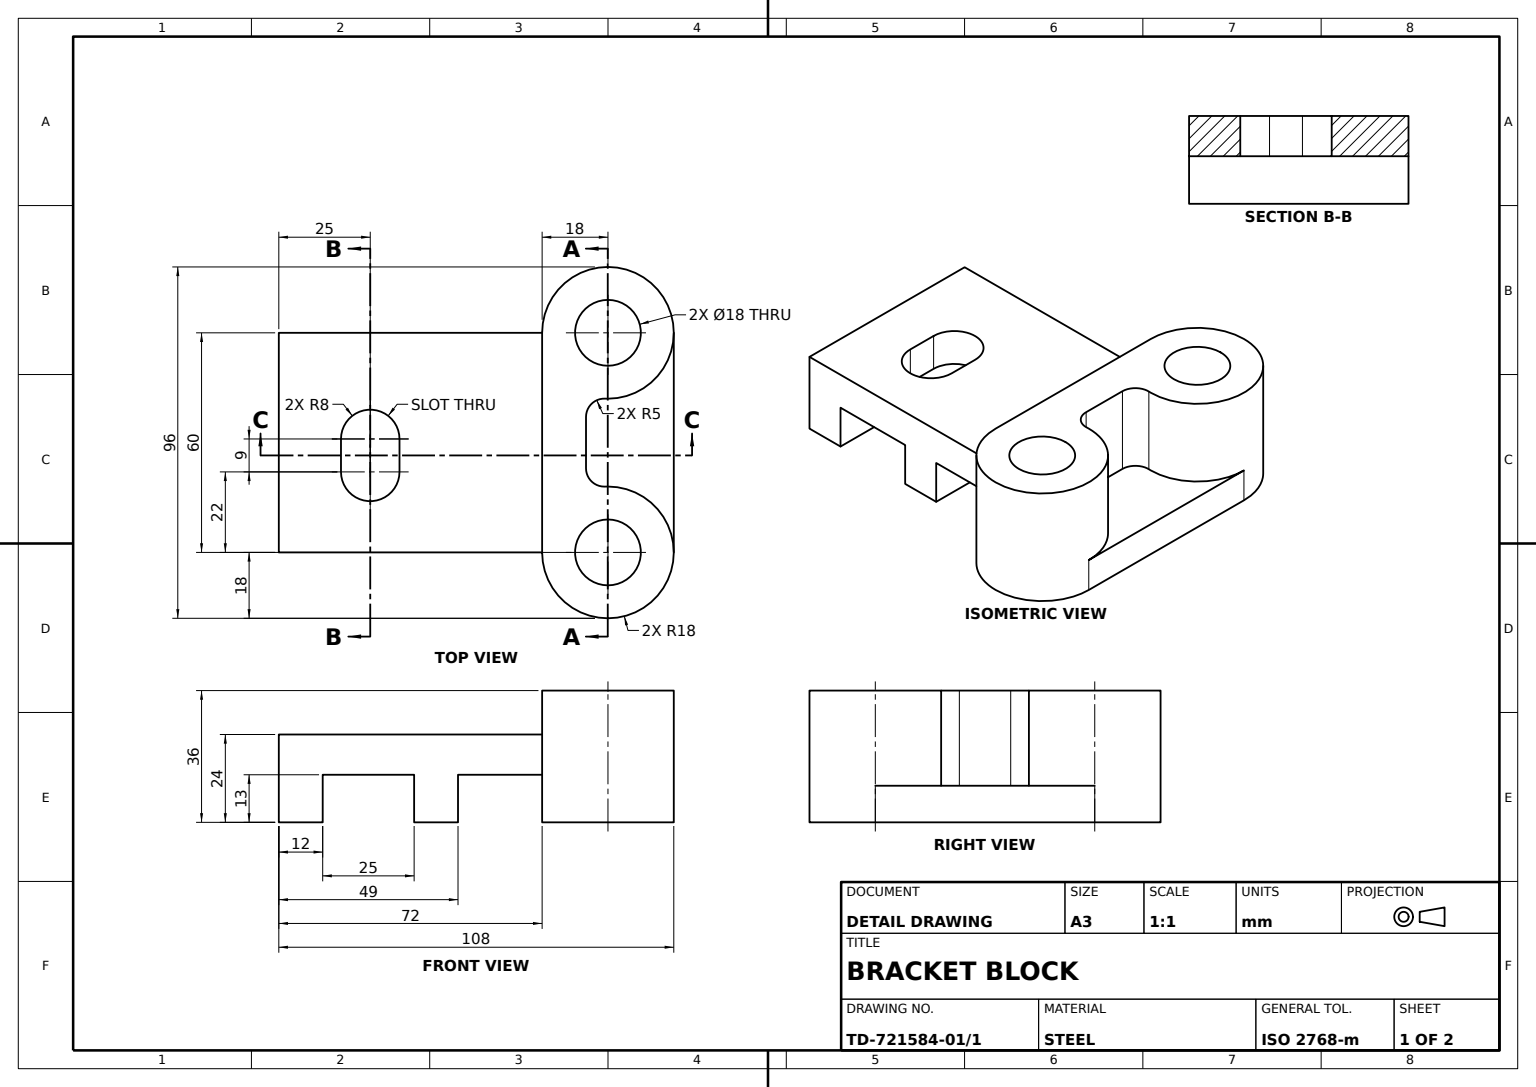
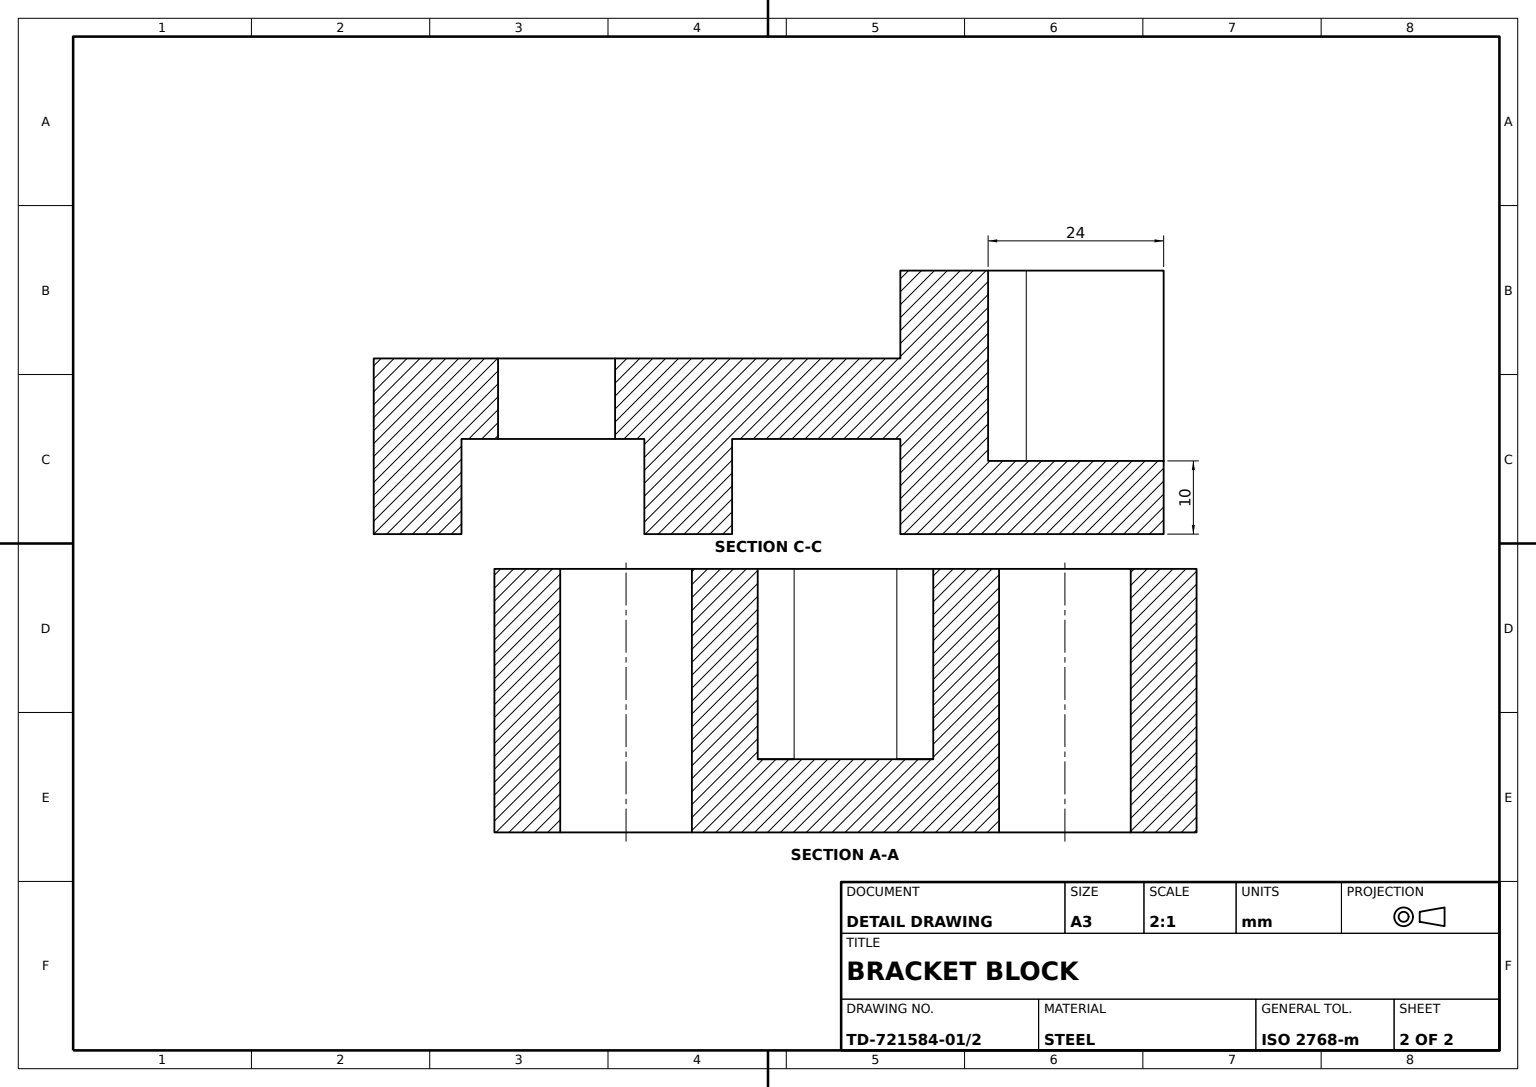
SolidWorks part; units mm, degrees
material "Plain Carbon Steel"
ref_plane "Front Plane" through (0, 0, 0) normal (0, 0, 1) x (1, 0, 0)
ref_plane "Top Plane" through (0, 0, 0) normal (0, 1, 0) x (1, 0, 0)
ref_plane "Right Plane" through (0, 0, 0) normal (1, 0, 0) x (0, 0, -1)
sketch "Base Block Profile Sketch" plane through (0, 0, 0) normal (0, 0, 1) x (1, 0, 0)
  line L0 (0, 0) -> (12, 0)
  line L1 (12, 0) -> (12, 13)
  line L2 (12, 13) -> (37, 13)
  line L3 (37, 13) -> (37, 0)
  line L4 (37, 0) -> (49, 0)
  line L5 (49, 0) -> (49, 13)
  line L6 (49, 13) -> (72, 13)
  line L7 (72, 13) -> (72, 24)
  line L8 (72, 24) -> (0, 24)
  line L9 (0, 24) -> (0, 0)
  dimension "D1" = 12
  dimension "D2" = 13
  dimension "D3" = 25
  dimension "D4" = 13
  dimension "D5" = 24
  dimension "D6" = 49
  dimension "D7" = 72
extrude "Base Block" add sketch "Base Block Profile Sketch" along normal blind 60
ref_plane "Lug Sketch Plane" through (0, 36, 0) normal (0, 1, 0) x (1, 0, 0)
sketch "Twin Lug Profile Sketch" plane through (0, 36, 0) normal (0, 1, 0) x (1, 0, 0)
  line L0 (72, -30) -> (72, 0) construction
  line L3 (72, -60) -> (72, 0) construction
  line L4 (72, 0) -> (0, 0) construction
  line L5 (72, 0) -> (90, 0) construction
  line L6 (72, -30) -> (72, -60) construction
  line L7 (72, -60) -> (90, -60) construction
  line L8 (72, 0) -> (72, -60)
  line L9 (84, -22.9783) -> (84, -37.0217)
  line L11 (84, 0) -> (84, -60) construction
  arc A0 (89.2174, -17.983) -> (72, 0) centre (90, 0) ccw
  arc A1 (72, -60) -> (89.2174, -42.017) centre (90, -60) ccw
  circle A2 centre (90, 0) radius 9
  circle A3 centre (90, -60) radius 9
  arc A4 (89.2174, -17.983) -> (84, -22.9783) centre (89, -22.9783) ccw
  arc A5 (84, -37.0217) -> (89.2174, -42.017) centre (89, -37.0217) ccw
  dimension "D1" = 36
  dimension "D2" = 36
  dimension "D6" = 18
  dimension "D7" = 18
  dimension "D9" = 5
  dimension "D10" = 5
  dimension "D5" = 60
  dimension "D8" = 12
extrude "Twin Lugs" add sketch "Twin Lug Profile Sketch" against normal blind 36
ref_plane "Lug Web Plane" through (0, 0, 0) normal (0, 1, 0) x (1, 0, 0)
sketch "Lug Web Profile Sketch" plane through (0, 0, 0) normal (0, 1, 0) x (1, 0, 0)
  line L0 (108, 0) -> (108, -60)
  line L1 (84, -22.9783) -> (84, -37.0217)
  arc A0 (89.2174, -17.983) -> (72, 0) centre (90, 0) ccw construction
  arc A1 (72, -60) -> (89.2174, -42.017) centre (90, -60) ccw construction
  arc A2 (89.2174, -17.983) -> (108, 0) centre (90, 0) ccw
  arc A3 (108, -60) -> (88.4299, -42.0686) centre (90, -60) ccw
  arc A4 (84, -22.9783) -> (89.2174, -17.983) centre (89, -22.9783) cw
  arc A5 (84, -37.0217) -> (90, -42) centre (88.9994, -37.1011) ccw
  dimension "D1" = 5
extrude "Lug Web" add sketch "Lug Web Profile Sketch" along normal blind 10 contours L1 A5 A3 L0 A2 A4
sketch "Mounting Slot Sketch" plane through (0, 24, 0) normal (0, 1, 0) x (1, 0, 0)
  line L0 (25, -29) -> (25, -38) construction
  line L1 (33, -29) -> (33, -38)
  line L2 (17, -29) -> (17, -38)
  arc A0 (33, -29) -> (17, -29) centre (25, -29) ccw
  arc A1 (17, -38) -> (33, -38) centre (25, -38) ccw
  point P2 (25, -33.5)
  dimension "D2" = 8
  dimension "D1" = 9
  dimension "D3" = 22
  dimension "D4" = 25
extrude "Mounting Slot 9mm" cut sketch "Mounting Slot Sketch" against normal through all
